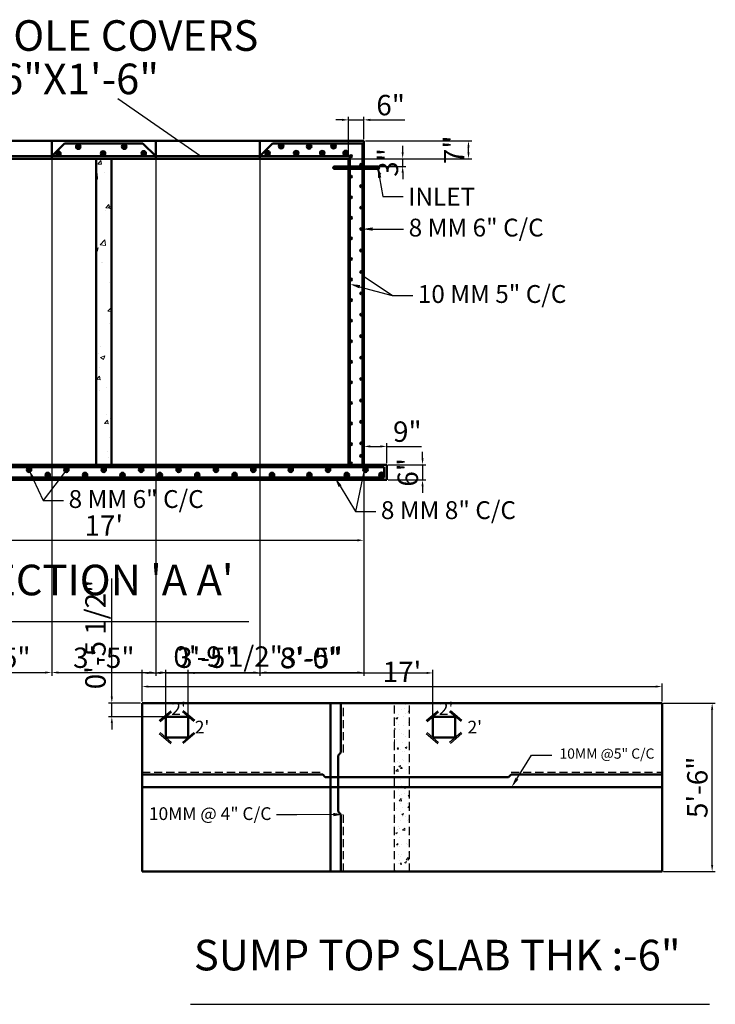
# Model space of a CAD drawing. Units: inches. Extents: x 2473 to 3272, y 1467 to 1853.
# Tile 2 of 3: x 2638 to 2911, y 1467 to 1853. Entities that reach past the tile are written whole.
import ezdxf
from ezdxf import colors
from ezdxf.entities.mleader import LeaderData, LeaderLine
from ezdxf.math import Vec2, Vec3

# ---------------------------------------------------------------- set-up
doc = ezdxf.new("R2010")
doc.units = ezdxf.units.IN
doc.header["$PDMODE"] = 36
doc.linetypes.add('HIDDEN', pattern=[9.525, 6.35, -3.175])
for name, color, linetype, lineweight in [('S-ANNO-DIMS', 2, 'Continuous', 25), ('S-ANNO-TEXT', 7, 'Continuous', 25), ('S-CONC', 7, 'Continuous', 50), ('S-CONC-HIDN', 4, 'HIDDEN', 25), ('S-CONC-PATT', 8, 'Continuous', 13), ('S-REIN', 3, 'Continuous', 35)]:
    doc.layers.add(name, color=color, linetype=linetype, lineweight=lineweight)
doc.styles.get("Standard").update_dxf_attribs({"font": '@Yu Gothic UI Semibold.ttf'})
doc.dimstyles.new('ISO-25', dxfattribs={"dimtxt": 8, "dimasz": 2.5, "dimexe": 1.25, "dimexo": 0.625, "dimtad": 1, "dimdec": 1, "dimlunit": 3, "dimtxsty": 'Standard', "dimcen": 2.5, "dimadec": 0, "dimazin": 0, "dimtfac": 1, "dimtdec": 1, "dimtmove": 0, "dimatfit": 3, "dimfxl": 1, "dimarcsym": 0})

# ---------------------------------------------------------------- blocks, each defined once
blk = doc.blocks.new('*D6')
at = {"layer": 'Defpoints', "color": 0, "transparency": 16777216}
for p in [(2890.46, 1591.69), (2686.46, 1585.17), (2890.46, 1585.17)]:
    blk.add_point(p, dxfattribs=at)
at = {"layer": 'S-ANNO-DIMS', "color": 0, "lineweight": -2, "transparency": 16777216}
for p, q in [((2686.46, 1585.79), (2686.46, 1592.94)), ((2688.96, 1591.69), (2887.96, 1591.69)), ((2890.46, 1585.79), (2890.46, 1592.94))]:
    blk.add_line(p, q, dxfattribs=at)
at = {"layer": 'S-ANNO-DIMS', "color": 0, "transparency": 16777216}
for points in [[(2688.96, 1592.11), (2688.96, 1591.27), (2686.46, 1591.69)], [(2887.96, 1592.11), (2887.96, 1591.27), (2890.46, 1591.69)]]:
    blk.add_solid(points, dxfattribs=at)
at = {"layer": 'S-ANNO-DIMS', "color": 0, "transparency": 16777216, "insert": (2788.46, 1596.41), "char_height": 8, "attachment_point": 5}
blk.add_mtext("17'", dxfattribs=at)
blk = doc.blocks.new('*D7')
at = {"layer": 'Defpoints', "color": 0, "transparency": 16777216}
for p in [(2890.46, 1585.17), (2910.13, 1585.17), (2890.46, 1519.17)]:
    blk.add_point(p, dxfattribs=at)
at = {"layer": 'S-ANNO-DIMS', "color": 0, "lineweight": -2, "transparency": 16777216}
for p, q in [((2891.09, 1585.17), (2911.38, 1585.17)), ((2910.13, 1521.67), (2910.13, 1582.67)), ((2891.09, 1519.17), (2911.38, 1519.17))]:
    blk.add_line(p, q, dxfattribs=at)
at = {"layer": 'S-ANNO-DIMS', "color": 0, "transparency": 16777216}
for points in [[(2909.71, 1582.67), (2910.54, 1582.67), (2910.13, 1585.17)], [(2909.71, 1521.67), (2910.54, 1521.67), (2910.13, 1519.17)]]:
    blk.add_solid(points, dxfattribs=at)
at = {"layer": 'S-ANNO-DIMS', "color": 0, "transparency": 16777216, "insert": (2905.36, 1552.17), "char_height": 8, "attachment_point": 5, "rotation": 90}
blk.add_mtext('5\'-6"', dxfattribs=at)
blk = doc.blocks.new('*D8')
at = {"layer": 'Defpoints', "color": 0, "transparency": 16777216}
for p in [(2569.47, 1678.69), (2773.47, 1678.69), (2773.47, 1649.05)]:
    blk.add_point(p, dxfattribs=at)
at = {"layer": 'S-ANNO-DIMS', "color": 0, "lineweight": -2, "transparency": 16777216}
for p, q in [((2569.47, 1678.06), (2569.47, 1647.8)), ((2773.47, 1678.06), (2773.47, 1647.8)), ((2571.97, 1649.05), (2770.97, 1649.05))]:
    blk.add_line(p, q, dxfattribs=at)
at = {"layer": 'S-ANNO-DIMS', "color": 0, "transparency": 16777216}
for points in [[(2571.97, 1649.47), (2571.97, 1648.63), (2569.47, 1649.05)], [(2770.97, 1649.47), (2770.97, 1648.63), (2773.47, 1649.05)]]:
    blk.add_solid(points, dxfattribs=at)
at = {"layer": 'S-ANNO-DIMS', "color": 0, "transparency": 16777216, "insert": (2671.47, 1653.76), "char_height": 8, "attachment_point": 5}
blk.add_mtext("17'", dxfattribs=at)
blk = doc.blocks.new('*D9')
at = {"layer": 'Defpoints', "color": 0, "transparency": 16777216}
for p in [(2782.47, 1678.69), (2782.47, 1672.69), (2796.52, 1672.69)]:
    blk.add_point(p, dxfattribs=at)
at = {"layer": 'S-ANNO-DIMS', "color": 0, "lineweight": -2, "transparency": 16777216}
for p, q in [((2796.52, 1681.19), (2796.52, 1683.69)), ((2783.09, 1678.69), (2797.77, 1678.69)), ((2796.52, 1678.69), (2796.52, 1672.69)), ((2783.09, 1672.69), (2797.77, 1672.69)), ((2796.52, 1670.19), (2796.52, 1667.69))]:
    blk.add_line(p, q, dxfattribs=at)
at = {"layer": 'S-ANNO-DIMS', "color": 0, "transparency": 16777216}
for points in [[(2796.1, 1681.19), (2796.94, 1681.19), (2796.52, 1678.69)], [(2796.1, 1670.19), (2796.94, 1670.19), (2796.52, 1672.69)]]:
    blk.add_solid(points, dxfattribs=at)
at = {"layer": 'S-ANNO-DIMS', "color": 0, "transparency": 16777216, "insert": (2791.76, 1675.69), "char_height": 8, "attachment_point": 5, "rotation": 90}
blk.add_mtext('6"', dxfattribs=at)
blk = doc.blocks.new('*D10')
at = {"layer": 'Defpoints', "color": 0, "transparency": 16777216}
for p in [(2782.47, 1685.86), (2773.47, 1678.69), (2782.47, 1678.69)]:
    blk.add_point(p, dxfattribs=at)
at = {"layer": 'S-ANNO-DIMS', "color": 0, "lineweight": -2, "transparency": 16777216}
for p, q in [((2773.47, 1679.31), (2773.47, 1687.11)), ((2775.97, 1685.86), (2779.97, 1685.86)), ((2782.47, 1679.31), (2782.47, 1687.11)), ((2782.47, 1685.86), (2796.13, 1685.86))]:
    blk.add_line(p, q, dxfattribs=at)
at = {"layer": 'S-ANNO-DIMS', "color": 0, "transparency": 16777216}
for points in [[(2775.97, 1686.27), (2775.97, 1685.44), (2773.47, 1685.86)], [(2779.97, 1686.27), (2779.97, 1685.44), (2782.47, 1685.86)]]:
    blk.add_solid(points, dxfattribs=at)
at = {"layer": 'S-ANNO-DIMS', "color": 0, "transparency": 16777216, "insert": (2790.55, 1690.62), "char_height": 8, "attachment_point": 5}
blk.add_mtext('9"', dxfattribs=at)
blk = doc.blocks.new('*D15')
at = {"layer": 'Defpoints', "color": 0, "transparency": 16777216}
for p in [(2773.47, 1813.91), (2773.47, 1805.69), (2767.47, 1798.69)]:
    blk.add_point(p, dxfattribs=at)
at = {"layer": 'S-ANNO-DIMS', "color": 0, "lineweight": -2, "transparency": 16777216}
for p, q in [((2767.47, 1799.31), (2767.47, 1815.16)), ((2773.47, 1806.31), (2773.47, 1815.16)), ((2764.97, 1813.91), (2762.47, 1813.91)), ((2767.47, 1813.91), (2773.47, 1813.91)), ((2775.97, 1813.91), (2789.54, 1813.91))]:
    blk.add_line(p, q, dxfattribs=at)
at = {"layer": 'S-ANNO-DIMS', "color": 0, "transparency": 16777216}
for points in [[(2764.97, 1814.33), (2764.97, 1813.49), (2767.47, 1813.91)], [(2775.97, 1814.33), (2775.97, 1813.49), (2773.47, 1813.91)]]:
    blk.add_solid(points, dxfattribs=at)
at = {"layer": 'S-ANNO-DIMS', "color": 0, "transparency": 16777216, "insert": (2784, 1818.67), "char_height": 8, "attachment_point": 5}
blk.add_mtext('6"', dxfattribs=at)
blk = doc.blocks.new('*D16')
at = {"layer": 'Defpoints', "color": 0, "transparency": 16777216}
for p in [(2773.47, 1805.69), (2814.54, 1805.69), (2767.47, 1798.69)]:
    blk.add_point(p, dxfattribs=at)
at = {"layer": 'S-ANNO-DIMS', "color": 0, "lineweight": -2, "transparency": 16777216}
for p, q in [((2774.09, 1805.69), (2815.79, 1805.69)), ((2814.54, 1801.19), (2814.54, 1803.19)), ((2768.09, 1798.69), (2815.79, 1798.69))]:
    blk.add_line(p, q, dxfattribs=at)
at = {"layer": 'S-ANNO-DIMS', "color": 0, "transparency": 16777216}
for points in [[(2814.13, 1803.19), (2814.96, 1803.19), (2814.54, 1805.69)], [(2814.13, 1801.19), (2814.96, 1801.19), (2814.54, 1798.69)]]:
    blk.add_solid(points, dxfattribs=at)
at = {"layer": 'S-ANNO-DIMS', "color": 0, "transparency": 16777216, "insert": (2809.92, 1802.19), "char_height": 8, "attachment_point": 5, "rotation": 90}
blk.add_mtext('7"', dxfattribs=at)
blk = doc.blocks.new('*D17')
at = {"layer": 'Defpoints', "color": 0, "transparency": 16777216}
for p in [(2767.47, 1798.69), (2767.47, 1795.69), (2788.72, 1798.69)]:
    blk.add_point(p, dxfattribs=at)
at = {"layer": 'S-ANNO-DIMS', "color": 0, "lineweight": -2, "transparency": 16777216}
for p, q in [((2788.72, 1801.19), (2788.72, 1803.69)), ((2768.09, 1798.69), (2789.97, 1798.69)), ((2768.09, 1795.69), (2789.97, 1795.69)), ((2788.72, 1795.69), (2788.72, 1798.69)), ((2788.72, 1793.19), (2788.72, 1790.69))]:
    blk.add_line(p, q, dxfattribs=at)
at = {"layer": 'S-ANNO-DIMS', "color": 0, "transparency": 16777216}
for points in [[(2788.3, 1801.19), (2789.13, 1801.19), (2788.72, 1798.69)], [(2788.3, 1793.19), (2789.13, 1793.19), (2788.72, 1795.69)]]:
    blk.add_solid(points, dxfattribs=at)
at = {"layer": 'S-ANNO-DIMS', "color": 0, "transparency": 16777216, "insert": (2783.96, 1797.19), "char_height": 8, "attachment_point": 5, "rotation": 90}
blk.add_mtext('3"', dxfattribs=at)
blk = doc.blocks.new('REBAR-SECTION-SMALL')
h = blk.add_hatch(color=256)
h.dxf.hatch_style = 1
h.paths.add_polyline_path([(2579.2, 1800.19, 1), (2578.2, 1800.19, 1)])
blk.add_circle((2578.7, 1800.19), 0.5)
blk = doc.blocks.new('REBAR-SECTION-LARGE')
h = blk.add_hatch(color=256)
h.dxf.hatch_style = 1
h.paths.add_polyline_path([(2652.73, 1800.68, 1), (2654.73, 1800.68, 1)])
blk.add_circle((2653.73, 1800.68), 1)
blk = doc.blocks.new('*D23')
at = {"layer": 'Defpoints', "color": 0, "transparency": 16777216}
for p in [(2610.27, 1805.69), (2651.07, 1805.69), (2651.07, 1597.2)]:
    blk.add_point(p, dxfattribs=at)
at = {"layer": 'S-ANNO-DIMS', "color": 0, "lineweight": -2, "transparency": 16777216}
for p, q in [((2610.27, 1805.06), (2610.27, 1595.95)), ((2651.07, 1805.06), (2651.07, 1595.95)), ((2612.77, 1597.2), (2648.57, 1597.2))]:
    blk.add_line(p, q, dxfattribs=at)
at = {"layer": 'S-ANNO-DIMS', "color": 0, "transparency": 16777216}
for points in [[(2612.77, 1597.61), (2612.77, 1596.78), (2610.27, 1597.2)], [(2648.57, 1597.61), (2648.57, 1596.78), (2651.07, 1597.2)]]:
    blk.add_solid(points, dxfattribs=at)
at = {"layer": 'S-ANNO-DIMS', "color": 0, "transparency": 16777216, "insert": (2630.67, 1601.96), "char_height": 8, "attachment_point": 5}
blk.add_mtext('3\'-5"', dxfattribs=at)
blk = doc.blocks.new('*D24')
at = {"layer": 'Defpoints', "color": 0, "transparency": 16777216}
for p in [(2651.07, 1805.69), (2691.87, 1805.69), (2691.87, 1597.2)]:
    blk.add_point(p, dxfattribs=at)
at = {"layer": 'S-ANNO-DIMS', "color": 0, "lineweight": -2, "transparency": 16777216}
for p, q in [((2651.07, 1805.06), (2651.07, 1595.95)), ((2691.87, 1805.06), (2691.87, 1595.95)), ((2653.57, 1597.2), (2689.37, 1597.2))]:
    blk.add_line(p, q, dxfattribs=at)
at = {"layer": 'S-ANNO-DIMS', "color": 0, "transparency": 16777216}
for points in [[(2653.57, 1597.61), (2653.57, 1596.78), (2651.07, 1597.2)], [(2689.37, 1597.61), (2689.37, 1596.78), (2691.87, 1597.2)]]:
    blk.add_solid(points, dxfattribs=at)
at = {"layer": 'S-ANNO-DIMS', "color": 0, "transparency": 16777216, "insert": (2671.47, 1601.96), "char_height": 8, "attachment_point": 5}
blk.add_mtext('3\'-5"', dxfattribs=at)
blk = doc.blocks.new('*D25')
at = {"layer": 'Defpoints', "color": 0, "transparency": 16777216}
for p in [(2691.87, 1805.69), (2732.67, 1805.69), (2732.67, 1597.2)]:
    blk.add_point(p, dxfattribs=at)
at = {"layer": 'S-ANNO-DIMS', "color": 0, "lineweight": -2, "transparency": 16777216}
for p, q in [((2691.87, 1805.06), (2691.87, 1595.95)), ((2732.67, 1805.06), (2732.67, 1595.95)), ((2694.37, 1597.2), (2730.17, 1597.2))]:
    blk.add_line(p, q, dxfattribs=at)
at = {"layer": 'S-ANNO-DIMS', "color": 0, "transparency": 16777216}
for points in [[(2694.37, 1597.61), (2694.37, 1596.78), (2691.87, 1597.2)], [(2730.17, 1597.61), (2730.17, 1596.78), (2732.67, 1597.2)]]:
    blk.add_solid(points, dxfattribs=at)
at = {"layer": 'S-ANNO-DIMS', "color": 0, "transparency": 16777216, "insert": (2712.27, 1601.96), "char_height": 8, "attachment_point": 5}
blk.add_mtext('3\'-5"', dxfattribs=at)
blk = doc.blocks.new('*D26')
at = {"layer": 'Defpoints', "color": 0, "transparency": 16777216}
for p in [(2732.67, 1805.69), (2773.47, 1805.69), (2773.47, 1597.2)]:
    blk.add_point(p, dxfattribs=at)
at = {"layer": 'S-ANNO-DIMS', "color": 0, "lineweight": -2, "transparency": 16777216}
for p, q in [((2732.67, 1805.06), (2732.67, 1595.95)), ((2773.47, 1805.06), (2773.47, 1595.95)), ((2735.17, 1597.2), (2770.97, 1597.2))]:
    blk.add_line(p, q, dxfattribs=at)
at = {"layer": 'S-ANNO-DIMS', "color": 0, "transparency": 16777216}
for points in [[(2735.17, 1597.61), (2735.17, 1596.78), (2732.67, 1597.2)], [(2770.97, 1597.61), (2770.97, 1596.78), (2773.47, 1597.2)]]:
    blk.add_solid(points, dxfattribs=at)
at = {"layer": 'S-ANNO-DIMS', "color": 0, "transparency": 16777216, "insert": (2753.07, 1601.96), "char_height": 8, "attachment_point": 5}
blk.add_mtext('3\'-5"', dxfattribs=at)
blk = doc.blocks.new('*D27')
at = {"layer": 'Defpoints', "color": 0, "transparency": 16777216}
for p in [(2695.8, 1597.02), (2686.46, 1585.17), (2695.8, 1579.87)]:
    blk.add_point(p, dxfattribs=at)
at = {"layer": 'S-ANNO-DIMS', "color": 0, "lineweight": -2, "transparency": 16777216}
for p, q in [((2686.46, 1585.79), (2686.46, 1598.27)), ((2688.96, 1597.02), (2693.3, 1597.02)), ((2695.8, 1580.49), (2695.8, 1598.27)), ((2695.8, 1597.02), (2742.2, 1597.02))]:
    blk.add_line(p, q, dxfattribs=at)
at = {"layer": 'S-ANNO-DIMS', "color": 0, "transparency": 16777216}
for points in [[(2688.96, 1597.44), (2688.96, 1596.6), (2686.46, 1597.02)], [(2693.3, 1597.44), (2693.3, 1596.6), (2695.8, 1597.02)]]:
    blk.add_solid(points, dxfattribs=at)
at = {"layer": 'S-ANNO-DIMS', "color": 0, "transparency": 16777216, "insert": (2720.25, 1602.4), "char_height": 8, "attachment_point": 5}
blk.add_mtext('0\'-9 1/2"', dxfattribs=at)
blk = doc.blocks.new('*D28')
at = {"layer": 'Defpoints', "color": 0, "transparency": 16777216}
for p in [(2800.58, 1597.02), (2704.57, 1579.87), (2800.58, 1579.87)]:
    blk.add_point(p, dxfattribs=at)
at = {"layer": 'S-ANNO-DIMS', "color": 0, "lineweight": -2, "transparency": 16777216}
for p, q in [((2704.57, 1580.49), (2704.57, 1598.27)), ((2707.07, 1597.02), (2798.08, 1597.02)), ((2800.58, 1580.49), (2800.58, 1598.27))]:
    blk.add_line(p, q, dxfattribs=at)
at = {"layer": 'S-ANNO-DIMS', "color": 0, "transparency": 16777216}
for points in [[(2707.07, 1597.44), (2707.07, 1596.6), (2704.57, 1597.02)], [(2798.08, 1597.44), (2798.08, 1596.6), (2800.58, 1597.02)]]:
    blk.add_solid(points, dxfattribs=at)
at = {"layer": 'S-ANNO-DIMS', "color": 0, "transparency": 16777216, "insert": (2752.58, 1601.78), "char_height": 8, "attachment_point": 5}
blk.add_mtext('8\'-0"', dxfattribs=at)
blk = doc.blocks.new('*D29')
at = {"layer": 'Defpoints', "color": 0, "transparency": 16777216}
for p in [(2674.61, 1585.17), (2686.46, 1585.17), (2695.8, 1579.87)]:
    blk.add_point(p, dxfattribs=at)
at = {"layer": 'S-ANNO-DIMS', "color": 0, "lineweight": -2, "transparency": 16777216}
for p, q in [((2674.61, 1587.67), (2674.61, 1634.04)), ((2685.84, 1585.17), (2673.36, 1585.17)), ((2674.61, 1579.87), (2674.61, 1585.17)), ((2695.18, 1579.87), (2673.36, 1579.87)), ((2674.61, 1577.37), (2674.61, 1574.87))]:
    blk.add_line(p, q, dxfattribs=at)
at = {"layer": 'S-ANNO-DIMS', "color": 0, "transparency": 16777216}
for points in [[(2674.2, 1587.67), (2675.03, 1587.67), (2674.61, 1585.17)], [(2674.2, 1577.37), (2675.03, 1577.37), (2674.61, 1579.87)]]:
    blk.add_solid(points, dxfattribs=at)
at = {"layer": 'S-ANNO-DIMS', "color": 0, "transparency": 16777216, "insert": (2669.23, 1612.1), "char_height": 8, "attachment_point": 5, "rotation": 90}
blk.add_mtext('0\'-5 1/2"', dxfattribs=at)

msp = doc.modelspace()

# ---------------------------------------------------------------- hatches: boundary and pattern name
at = {"layer": 'S-CONC-PATT'}
h = msp.add_hatch(dxfattribs=at)
h.set_pattern_fill('AR-CONC', color=256, scale=0.09)
h.paths.add_polyline_path([(2674.47, 1798.69), (2668.47, 1798.69), (2668.47, 1678.69), (2674.47, 1678.69)])
h = msp.add_hatch(dxfattribs=at)
h.set_pattern_fill('AR-CONC', color=256, scale=0.04)
h.set_pattern_definition([(50, (107.626, -40.585), (7.287387, -0.637563), [0.762, -8.382]), (355, (107.626, -40.585), (-1.409737, 7.642274), [0.6096, -6.705623]), (100.45144, (108.233, -40.638), (5.87765, 7.00471), [0.6476, -7.12361]), (46.1842, (107.626, -38.553), (10.843162, -1.681693), [1.143, -12.573]), (96.63556, (108.529, -38.693), (9.496165, 9.897045), [0.9714, -10.685424]), (351.18415, (107.626, -38.553), (9.496165, 9.897045), [0.9144, -10.05839]), (21, (108.642, -39.061), (6.064576, -4.090608), [0.762, -8.382]), (326, (108.642, -39.061), (2.472081, 7.367519), [0.6096, -6.7056]), (71.45144, (109.147, -39.402), (8.536657, 3.27691), [0.6476, -7.123598]), (37.5, (107.6258, -40.5848), (0.1235441, 3.3822016), [0, -6.62432, 0, -6.8072, 0, -6.731]), (7.5, (107.626, -40.5848), (2.6727865, 4.007223), [0, -3.88112, 0, -6.47192, 0, -2.5654]), (327.5, (105.3602, -40.5848), (5.4236238, -0.2291498), [0, -2.54, 0, -7.9248, 0, -10.5156]), (317.5, (104.344, -40.585), (5.925167, 1.01706), [0, -3.302, 0, -5.26288, 0, -7.4676])])
h.paths.add_polyline_path([(2791.46, 1585.17), (2785.46, 1585.17), (2785.46, 1556.17), (2791.46, 1556.17)])
h.paths.add_polyline_path([(2791.46, 1556.17), (2785.46, 1556.17), (2785.46, 1552.17), (2791.46, 1552.17)])
h.paths.add_polyline_path([(2791.46, 1552.17), (2785.46, 1552.17), (2785.46, 1519.17), (2791.46, 1519.17)])

# ---------------------------------------------------------------- linework, layer by layer
at = {"layer": 'S-ANNO-DIMS'}
for p, q in [((2693.21, 1578.34), (2697.71, 1582.21)), ((2693.54, 1577.96), (2698.04, 1581.83)), ((2706.84, 1577.96), (2702.33, 1581.83)), ((2707.16, 1578.34), (2702.66, 1582.21)), ((2797.99, 1578.34), (2802.49, 1582.21)), ((2798.31, 1577.96), (2802.82, 1581.83)), ((2811.61, 1577.96), (2807.11, 1581.83)), ((2811.94, 1578.34), (2807.44, 1582.21)), ((2693.21, 1573.28), (2697.71, 1569.41)), ((2693.54, 1573.66), (2698.04, 1569.79)), ((2706.84, 1573.66), (2702.33, 1569.79)), ((2707.16, 1573.28), (2702.66, 1569.41)), ((2797.99, 1573.28), (2802.49, 1569.41)), ((2798.31, 1573.66), (2802.82, 1569.79)), ((2811.61, 1573.66), (2807.11, 1569.79)), ((2811.94, 1573.28), (2807.44, 1569.41))]:
    msp.add_line(p, q, dxfattribs=at)
at = {"layer": 'S-ANNO-TEXT'}
for p, q in [((2709.36, 1799.69), (2676.99, 1822.12)), ((2784.66, 1745.05), (2772.97, 1752.73)), ((2656.8, 1676.69), (2647.67, 1664.64)), ((2773.47, 1675.94), (2770.17, 1660.29)), ((2612.08, 1617.15), (2728.34, 1617.15)), ((2705.46, 1467.08), (2909.06, 1467.08))]:
    msp.add_line(p, q, dxfattribs=at)
at = {"layer": 'S-CONC'}
for p, q in [((2569.47, 1805.69), (2773.47, 1805.69)), ((2651.07, 1798.69), (2651.07, 1805.69)), ((2651.07, 1799.69), (2656.1, 1804.69)), ((2656.1, 1804.69), (2686.78, 1804.69)), ((2691.87, 1799.69), (2686.78, 1804.69)), ((2691.87, 1798.69), (2691.87, 1805.69)), ((2732.67, 1798.69), (2732.67, 1805.69)), ((2732.67, 1799.69), (2737.67, 1804.69)), ((2737.67, 1804.69), (2772.97, 1804.69)), ((2772.97, 1804.69), (2772.97, 1678.69)), ((2773.47, 1805.69), (2773.47, 1678.69)), ((2574.97, 1799.69), (2767.97, 1799.69)), ((2767.97, 1799.69), (2767.97, 1678.69)), ((2575.47, 1798.69), (2767.47, 1798.69)), ((2668.47, 1798.69), (2668.47, 1678.69)), ((2674.47, 1798.69), (2674.47, 1678.69)), ((2767.47, 1795.69), (2761.96, 1795.69)), ((2767.47, 1798.69), (2767.47, 1678.69)), ((2767.47, 1795.69), (2779.02, 1795.69)), ((2761.96, 1794.69), (2767.47, 1794.69)), ((2767.47, 1794.69), (2779.02, 1794.69)), ((2560.47, 1678.69), (2782.47, 1678.69)), ((2561.47, 1677.69), (2781.47, 1677.69)), ((2781.47, 1677.69), (2781.47, 1673.69)), ((2782.47, 1678.69), (2782.47, 1672.69)), ((2560.47, 1672.69), (2782.47, 1672.69)), ((2561.47, 1673.69), (2781.47, 1673.69)), ((2686.46, 1585.17), (2890.46, 1585.17)), ((2686.46, 1519.17), (2686.46, 1585.17)), ((2760.46, 1519.17), (2760.46, 1585.17)), ((2764.46, 1565.84), (2764.46, 1585.17)), ((2890.46, 1585.17), (2890.46, 1519.17)), ((2763.46, 1564.69), (2764.46, 1565.84)), ((2763.46, 1542.74), (2763.46, 1564.69)), ((2686.46, 1557.17), (2757.37, 1557.17)), ((2758.34, 1556.17), (2757.37, 1557.17)), ((2758.34, 1556.17), (2830.22, 1556.17)), ((2830.22, 1556.17), (2831.22, 1557.17)), ((2831.22, 1557.17), (2890.46, 1557.17)), ((2686.46, 1552.17), (2890.46, 1552.17)), ((2763.46, 1542.74), (2764.46, 1541.51)), ((2764.46, 1519.17), (2764.46, 1541.51)), ((2890.46, 1519.17), (2686.46, 1519.17))]:
    msp.add_line(p, q, dxfattribs=at)
for points in [[(2695.8, 1579.87), (2704.57, 1579.87), (2704.57, 1571.75), (2695.8, 1571.75)], [(2800.58, 1579.87), (2809.35, 1579.87), (2809.35, 1571.75), (2800.58, 1571.75)]]:
    msp.add_lwpolyline(points, close=True, dxfattribs=at)
for centre in [(2761.96, 1795.19), (2779.02, 1795.19)]:
    msp.add_circle(centre, 0.5, dxfattribs=at)
at = {"layer": 'S-CONC-HIDN', "ltscale": 0.5}
for p, q in [((2765.46, 1565.84), (2765.46, 1585.17)), ((2785.46, 1519.17), (2785.46, 1585.17)), ((2791.46, 1519.17), (2791.46, 1585.17)), ((2686.46, 1558.17), (2757.37, 1558.17)), ((2831.22, 1558.17), (2890.46, 1558.17)), ((2765.46, 1519.17), (2765.46, 1541.51))]:
    msp.add_line(p, q, dxfattribs=at)

# ---------------------------------------------------------------- block references
at = {"layer": 'S-REIN', "rotation": 180}
for name, p in [('REBAR-SECTION-LARGE', (5315.18, 3604.09)), ('REBAR-SECTION-LARGE', (5333.2, 3604.09)), ('REBAR-SECTION-LARGE', (5394.77, 3604.24)), ('REBAR-SECTION-LARGE', (5405.75, 3604.15)), ('REBAR-SECTION-LARGE', (5415.33, 3604.24)), ('REBAR-SECTION-LARGE', (5307.4, 3601.37)), ('REBAR-SECTION-LARGE', (5324.9, 3601.45)), ('REBAR-SECTION-LARGE', (5340.85, 3601.5)), ('REBAR-SECTION-LARGE', (5389.47, 3601.52)), ('REBAR-SECTION-LARGE', (5400.68, 3601.58)), ('REBAR-SECTION-LARGE', (5410.9, 3601.58)), ('REBAR-SECTION-LARGE', (5420.07, 3601.62)), ('REBAR-SECTION-SMALL', (5347.17, 3599.88)), ('REBAR-SECTION-SMALL', (5351.17, 3596.48)), ('REBAR-SECTION-SMALL', (5347.17, 3591.81)), ('REBAR-SECTION-SMALL', (5351.17, 3588.08)), ('REBAR-SECTION-SMALL', (5347.17, 3583.74)), ('REBAR-SECTION-SMALL', (5351.17, 3579.68)), ('REBAR-SECTION-SMALL', (5347.17, 3575.68)), ('REBAR-SECTION-SMALL', (5351.17, 3571.28)), ('REBAR-SECTION-SMALL', (5347.17, 3567.61)), ('REBAR-SECTION-SMALL', (5351.17, 3562.88)), ('REBAR-SECTION-SMALL', (5347.17, 3559.54)), ('REBAR-SECTION-SMALL', (5351.17, 3554.48)), ('REBAR-SECTION-SMALL', (5347.17, 3551.48)), ('REBAR-SECTION-SMALL', (5351.17, 3546.08)), ('REBAR-SECTION-SMALL', (5347.17, 3543.41)), ('REBAR-SECTION-SMALL', (5351.17, 3537.68)), ('REBAR-SECTION-SMALL', (5347.17, 3535.34)), ('REBAR-SECTION-SMALL', (5347.17, 3527.28)), ('REBAR-SECTION-SMALL', (5351.17, 3529.28)), ('REBAR-SECTION-SMALL', (5347.17, 3519.21)), ('REBAR-SECTION-SMALL', (5351.17, 3520.88)), ('REBAR-SECTION-SMALL', (5347.17, 3511.14)), ('REBAR-SECTION-SMALL', (5351.17, 3512.48)), ('REBAR-SECTION-SMALL', (5347.17, 3503.08)), ('REBAR-SECTION-SMALL', (5351.17, 3504.08)), ('REBAR-SECTION-SMALL', (5347.17, 3495.01)), ('REBAR-SECTION-SMALL', (5351.17, 3495.68)), ('REBAR-SECTION-SMALL', (5351.17, 3487.28)), ('REBAR-SECTION-SMALL', (5347.17, 3486.94)), ('REBAR-SECTION-SMALL', (5347.17, 3479.39)), ('REBAR-SECTION-SMALL', (5351.15, 3482.32)), ('REBAR-SECTION-LARGE', (5295.86, 3477.37)), ('REBAR-SECTION-LARGE', (5310.53, 3477.37)), ('REBAR-SECTION-LARGE', (5325.19, 3477.37)), ('REBAR-SECTION-LARGE', (5339.86, 3477.37)), ('REBAR-SECTION-LARGE', (5354.53, 3477.37)), ('REBAR-SECTION-LARGE', (5369.19, 3477.37)), ('REBAR-SECTION-LARGE', (5383.86, 3477.37)), ('REBAR-SECTION-LARGE', (5398.53, 3477.37)), ('REBAR-SECTION-LARGE', (5413.19, 3477.37)), ('REBAR-SECTION-LARGE', (5427.86, 3477.37)), ('REBAR-SECTION-LARGE', (5434.15, 3475.44)), ('REBAR-SECTION-LARGE', (5303.19, 3475.37)), ('REBAR-SECTION-LARGE', (5317.86, 3475.37)), ('REBAR-SECTION-LARGE', (5332.53, 3475.37)), ('REBAR-SECTION-LARGE', (5347.19, 3475.37)), ('REBAR-SECTION-LARGE', (5361.86, 3475.37)), ('REBAR-SECTION-LARGE', (5376.53, 3475.37)), ('REBAR-SECTION-LARGE', (5391.19, 3475.37)), ('REBAR-SECTION-LARGE', (5405.86, 3475.37)), ('REBAR-SECTION-LARGE', (5420.53, 3475.37))]:
    msp.add_blockref(name, p, dxfattribs=at)

# ---------------------------------------------------------------- texts
at = {"layer": 'S-ANNO-DIMS'}
for p in [(2697.96, 1580.54), (2802.9, 1580.56), (2707.16, 1573.28), (2814.16, 1573.28)]:
    msp.add_text("2'", height=5, dxfattribs=at).set_placement(p)
at = {"layer": 'S-ANNO-TEXT'}
for s, p in [('MAN HOLE COVERS', (2585.29, 1840.99)), ('1\'-6"X1\'-6"', (2611.42, 1823.98)), ("SECTION 'A A'", (2617.57, 1627.47)), ('SUMP TOP SLAB THK :-6"', (2706.82, 1480.38))]:
    msp.add_text(s, height=12, dxfattribs=at).set_placement(p)

# ---------------------------------------------------------------- dimensions: what is measured, and where the dimension line sits
at = {"layer": 'S-ANNO-DIMS'}
for base, p1, p2, override, picture, middle in [((2773.47, 1813.91), (2767.47, 1798.69), (2773.47, 1805.69), {"dimclrd": 0, "dimclre": 0, "dimclrt": 0}, '*D15', (2784, 1818.67)), ((2651.07, 1597.2), (2610.27, 1805.69), (2651.07, 1805.69), {"dimdec": 1, "dimlfac": 1, "dimrnd": 0, "dimzin": 1, "dimdsep": 46, "dimlunit": 4, "dimfrac": 2}, '*D23', (2630.67, 1601.96)), ((2691.87, 1597.2), (2651.07, 1805.69), (2691.87, 1805.69), {"dimdec": 1, "dimlfac": 1, "dimrnd": 0, "dimzin": 1, "dimdsep": 46, "dimlunit": 4, "dimfrac": 2}, '*D24', (2671.47, 1601.96)), ((2732.67, 1597.2), (2691.87, 1805.69), (2732.67, 1805.69), {"dimdec": 1, "dimlfac": 1, "dimrnd": 0, "dimzin": 1, "dimdsep": 46, "dimlunit": 4, "dimfrac": 2}, '*D25', (2712.27, 1601.96)), ((2773.47, 1597.2), (2732.67, 1805.69), (2773.47, 1805.69), {"dimdec": 1, "dimlfac": 1, "dimrnd": 0, "dimzin": 1, "dimdsep": 46, "dimlunit": 4, "dimfrac": 2}, '*D26', (2753.07, 1601.96)), ((2782.47, 1685.86), (2773.47, 1678.69), (2782.47, 1678.69), {"dimclrd": 0, "dimclre": 0, "dimclrt": 0}, '*D10', (2790.55, 1690.62)), ((2695.8, 1597.02), (2686.46, 1585.17), (2695.8, 1579.87), {"dimdec": 1, "dimlfac": 1, "dimrnd": 0, "dimzin": 1, "dimdsep": 46, "dimlunit": 4, "dimfrac": 2}, '*D27', (2720.25, 1602.4)), ((2800.58, 1597.02), (2704.57, 1579.87), (2800.58, 1579.87), {"dimdec": 1, "dimlfac": 1, "dimrnd": 0, "dimzin": 1, "dimdsep": 46, "dimlunit": 4, "dimfrac": 2}, '*D28', (2752.58, 1601.78)), ((2890.46, 1591.69), (2686.46, 1585.17), (2890.46, 1585.17), {"dimclrd": 0, "dimclre": 0, "dimclrt": 0}, '*D6', (2788.46, 1596.41))]:
    dim = msp.add_linear_dim(base=base, p1=p1, p2=p2, dimstyle='ISO-25', override=override, dxfattribs=at)
    dim.commit()
    dim.dimension.update_dxf_attribs({"geometry": picture, "text_midpoint": middle})
for base, p1, p2, angle, picture, middle in [((2814.54, 1805.69), (2767.47, 1798.69), (2773.47, 1805.69), 270, '*D16', (2814.54, 1802.19)), ((2788.72, 1798.69), (2767.47, 1795.69), (2767.47, 1798.69), 270, '*D17', (2788.72, 1797.19)), ((2796.52, 1672.69), (2782.47, 1678.69), (2782.47, 1672.69), 90, '*D9', (2796.52, 1675.69))]:
    dim = msp.add_linear_dim(base=base, p1=p1, p2=p2, angle=angle, dimstyle='ISO-25', override={"dimclrd": 0, "dimclre": 0, "dimclrt": 0}, dxfattribs=at)
    dim.commit()
    dim.dimension.update_dxf_attribs({"geometry": picture, "text_midpoint": middle, "dimtype": 160})
dim = msp.add_linear_dim(base=(2773.47, 1649.05), p1=(2569.47, 1678.69), p2=(2773.47, 1678.69), dimstyle='ISO-25', override={"dimclrd": 0, "dimclre": 0, "dimclrt": 0}, dxfattribs=at)
dim.commit()
dim.dimension.update_dxf_attribs({"geometry": '*D8', "text_midpoint": (2671.47, 1649.05), "dimtype": 160})
for base, p1, p2, override, picture, middle in [((2674.61, 1585.17), (2695.8, 1579.87), (2686.46, 1585.17), {"dimdec": 1, "dimlfac": 1, "dimrnd": 0, "dimzin": 1, "dimdsep": 46, "dimlunit": 4, "dimfrac": 2}, '*D29', (2669.23, 1612.1)), ((2910.13, 1585.17), (2890.46, 1519.17), (2890.46, 1585.17), {"dimclrd": 0, "dimclre": 0, "dimclrt": 0}, '*D7', (2905.36, 1552.17))]:
    dim = msp.add_linear_dim(base=base, p1=p1, p2=p2, angle=90, dimstyle='ISO-25', override=override, dxfattribs=at)
    dim.commit()
    dim.dimension.update_dxf_attribs({"geometry": picture, "text_midpoint": middle})

# ---------------------------------------------------------------- leaders
at = {"layer": 'S-ANNO-TEXT'}
ml = msp.add_multileader_mtext('Standard', dxfattribs=at)
ml.set_content('INLET', color=256)
ml.set_leader_properties()
ml.build(insert=Vec2(0, 0))
ctx = ml.context
ctx.base_point, ctx.char_height, ctx.plane_origin = Vec3(2788.91, 1783.8), 7, Vec3(2779.02, 1795.19)
notes = []
notes.append((ctx, [(0, (1, 1, 0), (2780.91, 1783.8), (1, 0), 8, [(0, [(2779.02, 1795.19)], 0, [])])]))
ctx.mtext.insert, ctx.mtext.flow_direction = Vec3(2790.91, 1787.3), 5
ml = msp.add_multileader_mtext('Standard', dxfattribs=at)
ml.set_content('8 MM 6" C/C', color=256)
ml.set_leader_properties()
ml.build(insert=Vec2(0, 0))
ctx = ml.context
ctx.base_point, ctx.char_height, ctx.plane_origin = Vec3(2789.07, 1771.09), 7, Vec3(2772.97, 1771.09)
notes.append((ctx, [(0, (1, 1, 0), (2781.07, 1771.09), (1, 0), 8, [(0, [(2772.97, 1771.09)], 0, [])])]))
ctx.mtext.insert, ctx.mtext.flow_direction = Vec3(2791.07, 1775.17), 5
ml = msp.add_multileader_mtext('Standard', dxfattribs=at)
ml.set_content('10 MM 5" C/C', color=256)
ml.set_leader_properties()
ml.build(insert=Vec2(0, 0))
ctx = ml.context
ctx.base_point, ctx.char_height, ctx.plane_origin = Vec3(2792.66, 1745.05), 7, Vec3(2767.97, 1749.53)
notes.append((ctx, [(0, (1, 1, 0), (2784.66, 1745.05), (1, 0), 8, [(0, [(2767.97, 1749.53)], 0, [])])]))
ctx.mtext.insert, ctx.mtext.flow_direction = Vec3(2794.66, 1749.13), 5
ml = msp.add_multileader_mtext('Standard', dxfattribs=at)
ml.set_content('8 MM 6" C/C', color=256)
ml.set_leader_properties()
ml.build(insert=Vec2(0, 0))
ctx = ml.context
ctx.base_point, ctx.char_height, ctx.plane_origin = Vec3(2655.67, 1664.64), 7, Vec3(2642.13, 1676.69)
notes.append((ctx, [(0, (1, 1, 0), (2647.67, 1664.64), (1, 0), 8, [(0, [(2642.13, 1676.69)], 0, [])])]))
ctx.mtext.insert, ctx.mtext.flow_direction = Vec3(2657.67, 1668.72), 5
ml = msp.add_multileader_mtext('Standard', dxfattribs=at)
ml.set_content('8 MM 8" C/C', color=256)
ml.set_leader_properties()
ml.build(insert=Vec2(0, 0))
ctx = ml.context
ctx.base_point, ctx.char_height, ctx.plane_origin = Vec3(2778.17, 1660.29), 7, Vec3(2762.1, 1673.69)
notes.append((ctx, [(0, (1, 1, 0), (2770.17, 1660.29), (1, 0), 8, [(0, [(2762.1, 1673.69)], 0, [])])]))
ctx.mtext.insert, ctx.mtext.flow_direction = Vec3(2780.17, 1664.37), 5
ml = msp.add_multileader_mtext('Standard', dxfattribs=at)
ml.set_content('10MM @5" C/C', color=(175, 217, 170))
ml.set_leader_properties()
ml.build(insert=Vec2(0, 0))
ctx = ml.context
ctx.base_point, ctx.plane_origin = Vec3(2847.3, 1564.81), Vec3(2831.42, 1552.17)
ctx.text_align_type = 2
notes.append((ctx, [(1, (1, 1, 0), (2839.3, 1564.81), (1, 0), 8, [(0, [(2831.42, 1552.17)], 0, [])])]))
ctx.mtext.insert, ctx.mtext.alignment, ctx.mtext.flow_direction = Vec3(2887.49, 1567.4), 3, 5
ml = msp.add_multileader_mtext('Standard', dxfattribs=at)
ml.set_content('10MM @ 4" C/C', color=(175, 217, 170))
ml.set_leader_properties()
ml.build(insert=Vec2(0, 0))
ctx = ml.context
ctx.base_point, ctx.char_height, ctx.plane_origin = Vec3(2684.05, 1541.44), 5, Vec3(2765.46, 1541.51)
ctx.text_align_type = 2
notes.append((ctx, [(0, (1, 1, 0), (2747.24, 1541.44), (-1, 0), 8, [(0, [(2765.46, 1541.51)], 0, [])])]))
ctx.mtext.insert, ctx.mtext.alignment, ctx.mtext.flow_direction = Vec3(2737.24, 1544.35), 3, 5
for ctx, leaders in notes:
    for number, flags, end, landing, length, lines in leaders:
        leader = LeaderData()
        leader.index, (leader.has_last_leader_line, leader.has_dogleg_vector, leader.attachment_direction) = number, flags
        leader.last_leader_point, leader.dogleg_vector, leader.dogleg_length = Vec3(end), Vec3(landing), length
        for number, points, colour, breaks in lines:
            line = LeaderLine()
            line.index, line.vertices, line.color, line.breaks = number, Vec3.list(points), colors.encode_raw_color(colour), breaks
            leader.lines.append(line)
        ctx.leaders.append(leader)

doc.saveas('drawing.dxf')
